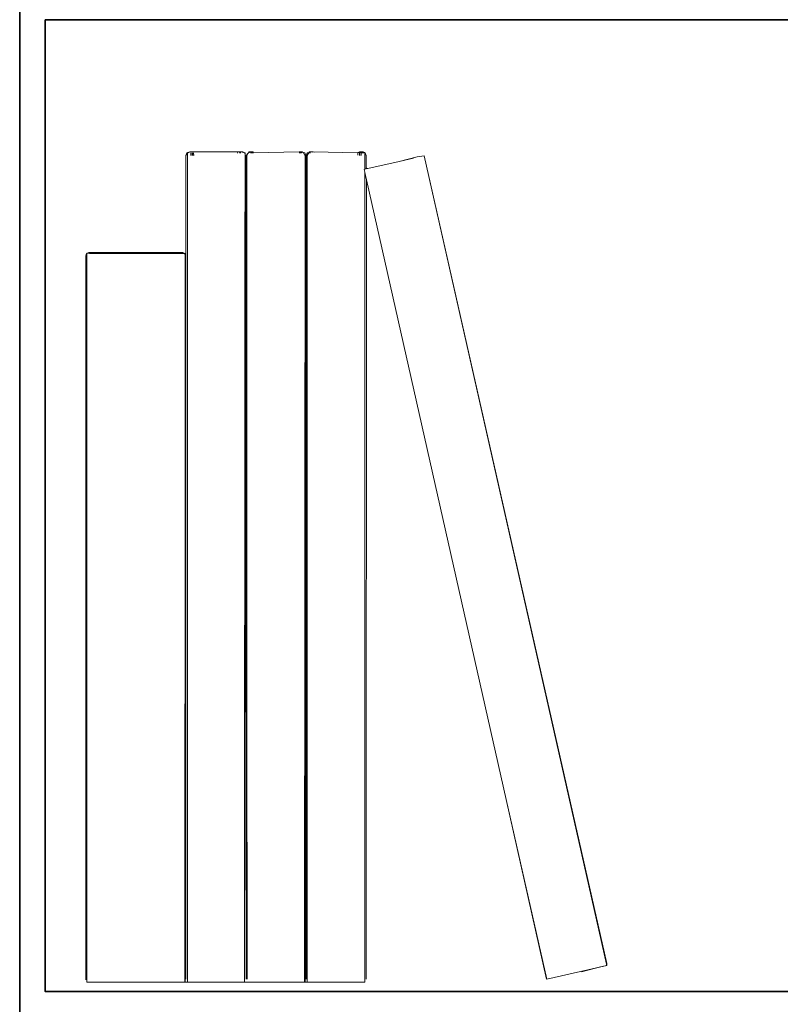
# Model space of a CAD drawing. Units: millimetres. Extents: x 446512 to 447461, y 70395 to 70610.
# Tile 5 of 39: x 446699.43 to 446714.29, y 70453.63 to 70472.88. Entities that reach past the tile are written whole.
import ezdxf

# ---------------------------------------------------------------- set-up
doc = ezdxf.new("R2010")
doc.units = ezdxf.units.MM
doc.layers.add('A-FURN', color=7, linetype='Continuous', lineweight=35)
doc.layers.add('A-FURN-DECO', color=8, linetype='Continuous', lineweight=13)

# ---------------------------------------------------------------- blocks, each defined once
blk = doc.blocks.new('DECO-VASE-C')
for p, q in [((1.958, 16.16), (1.977, 16.215)), ((1.977, 16.202), (1.958, 16.16)), ((1.977, 16.215), (1.982, 16.215)), ((1.977, 16.215), (1.977, 16.202)), ((1.982, 16.215), (1.977, 16.202)), ((1.977, 16.202), (1.977, 16.17)), ((1.982, 16.215), (1.989, 16.215)), ((1.989, 16.215), (1.988, 0)), ((1.989, 16.215), (1.997, 16.218)), ((1.997, 16.218), (2.035, 16.233)), ((2.016, 16.22), (1.997, 16.218)), ((1.997, 16.218), (2.009, 16.215)), ((2.019, 16.221), (2.016, 16.22)), ((3.07, 16.233), (2.035, 16.233)), ((2.054, 16.161), (2.053, 16.215)), ((2.058, 16.161), (2.058, 16.215)), ((2.088, 16.215), (2.094, 16.163)), ((2.088, 16.163), (2.088, 16.215)), ((2.088, 16.215), (2.09, 16.163)), ((2.106, 16.215), (2.11, 16.164)), ((2.969, 16.21), (2.969, 16.215)), ((2.976, 16.215), (2.969, 16.215)), ((2.999, 16.212), (2.999, 16.215)), ((3.004, 16.215), (3.004, 16.212)), ((3.034, 16.215), (3.004, 16.215)), ((3.058, 16.224), (3.11, 16.215)), ((3.07, 16.233), (3.111, 16.215)), ((3.111, 16.215), (3.11, 16.215)), ((3.114, 16.16), (3.111, 16.215)), ((3.115, 16.215), (3.111, 16.215)), ((3.114, 16.16), (3.115, 16.215)), ((3.133, 16.16), (3.177, 16.207)), ((3.152, 16.16), (3.177, 16.207)), ((3.177, 16.207), (3.184, 16.215)), ((3.184, 16.215), (3.19, 16.233)), ((3.184, 16.215), (3.23, 16.225)), ((3.27, 16.233), (3.19, 16.233)), ((3.221, 16.215), (3.263, 16.215)), ((3.263, 16.218), (3.263, 16.215)), ((3.263, 16.215), (3.281, 16.216)), ((3.281, 16.216), (3.27, 16.233)), ((3.281, 16.216), (4.174, 16.232)), ((4.171, 16.215), (4.179, 16.215)), ((4.176, 16.233), (4.174, 16.232)), ((4.178, 16.232), (4.176, 16.233)), ((4.178, 16.232), (4.232, 16.233)), ((4.179, 16.215), (4.179, 16.217)), ((4.209, 16.215), (4.179, 16.215)), ((4.209, 16.215), (4.196, 16.222)), ((4.214, 16.215), (4.209, 16.215)), ((4.212, 16.227), (4.224, 16.225)), ((4.224, 16.225), (4.214, 16.215)), ((4.232, 16.233), (4.224, 16.225)), ((4.224, 16.225), (4.249, 16.221)), ((4.232, 16.233), (4.249, 16.221)), ((4.249, 16.221), (4.258, 16.215)), ((4.249, 16.221), (4.285, 16.215)), ((4.283, 16.171), (4.258, 16.215)), ((4.283, 16.171), (4.285, 16.17)), ((4.29, 16.16), (4.283, 16.171)), ((4.309, 16.16), (4.285, 16.215)), ((4.309, 16.16), (4.327, 16.215)), ((4.332, 16.215), (4.309, 16.16)), ((4.327, 16.215), (4.332, 16.215)), ((4.327, 16.16), (4.36, 16.215)), ((4.332, 16.215), (4.363, 16.22)), ((4.36, 16.215), (4.332, 16.215)), ((4.36, 16.215), (4.363, 16.22)), ((4.396, 16.215), (4.36, 16.215)), ((4.363, 16.22), (4.37, 16.233)), ((4.363, 16.22), (4.384, 16.223)), ((4.439, 16.232), (4.37, 16.233)), ((4.438, 16.212), (4.438, 16.215)), ((4.442, 16.233), (4.439, 16.232)), ((4.439, 16.232), (4.444, 16.232)), ((4.442, 16.233), (4.444, 16.232)), ((4.442, 16.212), (4.442, 16.215)), ((4.444, 16.232), (5.319, 16.215)), ((4.469, 16.211), (4.47, 16.215)), ((5.319, 16.215), (5.317, 16.165)), ((5.319, 16.215), (5.322, 16.217)), ((5.322, 16.217), (5.351, 16.233)), ((5.322, 16.217), (5.35, 16.216)), ((5.35, 16.216), (5.348, 16.163)), ((5.351, 16.233), (5.35, 16.216)), ((5.35, 16.216), (5.354, 16.216)), ((5.351, 16.233), (5.354, 16.216)), ((5.383, 16.215), (5.351, 16.233)), ((5.351, 16.233), (5.422, 16.233)), ((5.351, 16.233), (5.398, 16.222)), ((5.403, 16.224), (5.351, 16.233)), ((5.354, 16.216), (5.352, 16.163)), ((5.354, 16.216), (5.355, 16.163)), ((5.354, 16.216), (5.383, 16.215)), ((5.383, 16.215), (5.386, 16.215)), ((5.383, 16.215), (5.384, 16.215)), ((5.384, 16.161), (5.384, 16.215)), ((5.384, 16.161), (5.386, 16.215)), ((5.384, 16.215), (5.386, 16.215)), ((5.386, 16.215), (5.433, 16.215)), ((5.386, 16.215), (5.388, 16.215)), ((5.388, 16.215), (5.398, 16.222)), ((5.398, 16.222), (5.4, 16.222)), ((5.4, 16.222), (5.403, 16.224)), ((5.4, 16.222), (5.433, 16.215)), ((5.405, 16.224), (5.403, 16.224)), ((5.405, 16.224), (5.422, 16.233)), ((5.449, 16.217), (5.405, 16.224)), ((5.449, 16.217), (5.422, 16.233)), ((5.433, 16.215), (5.449, 16.217)), ((5.453, 16.215), (5.449, 16.217)), ((5.453, 16.215), (5.453, 15.894)), ((5.465, 16.215), (5.453, 16.215)), ((5.465, 16.215), (5.484, 16.16)), ((5.465, 16.17), (5.465, 16.215)), ((1.958, 0.055), (1.958, 16.16)), ((3.114, 16.16), (3.113, 13.969)), ((3.133, 0.055), (3.114, 16.16)), ((3.152, 3.273), (3.133, 16.16)), ((3.133, 16.16), (3.153, 0.055)), ((3.152, 3.273), (3.152, 16.16)), ((4.279, 0), (4.29, 16.16)), ((4.285, 0), (4.309, 16.16)), ((4.29, 0), (4.309, 16.16)), ((4.309, 0.055), (4.309, 16.16)), ((4.309, 16.16), (4.327, 0.012)), ((4.331, 0.004), (4.327, 16.16)), ((5.484, 16.16), (5.484, 15.909)), ((5.516, 15.905), (6.127, 16.043)), ((6.127, 16.043), (6.476, 16.134)), ((6.127, 16.043), (6.409, 16.107)), ((6.614, 16.153), (6.476, 16.134)), ((6.615, 16.153), (6.614, 16.153)), ((6.614, 16.153), (10.177, 0.349)), ((10.188, 0.362), (6.615, 16.153)), ((5.442, 15.889), (5.453, 15.894)), ((5.442, 15.889), (5.454, 15.891)), ((5.453, 15.838), (5.442, 15.889)), ((5.453, 15.894), (5.484, 15.909)), ((5.453, 15.894), (5.454, 15.891)), ((5.453, 15.838), (5.453, 15.829)), ((5.453, 15.829), (5.454, 0)), ((5.485, 15.688), (5.453, 15.829)), ((5.516, 15.905), (5.454, 15.891)), ((5.492, 15.912), (5.484, 15.909)), ((5.484, 15.909), (5.484, 15.903)), ((5.492, 15.912), (5.516, 15.905)), ((5.485, 15.688), (5.484, 0.055)), ((5.485, 15.688), (8.218, 3.572)), ((0, 14.202), (0.014, 14.248)), ((0.014, 14.248), (0.018, 14.248)), ((0.014, 14.248), (0.014, 14.237)), ((0.018, 14.248), (0.014, 14.237)), ((0.018, 14.248), (0.023, 14.248)), ((0.023, 14.248), (0.029, 14.25)), ((0.023, 0), (0.023, 14.248)), ((0.029, 14.25), (0.06, 14.263)), ((0.029, 14.25), (0.066, 14.256)), ((0.074, 14.248), (0.029, 14.25)), ((0.06, 14.263), (0.104, 14.263)), ((0.066, 14.256), (0.06, 14.263)), ((0.066, 14.256), (0.104, 14.263)), ((0.074, 14.248), (0.066, 14.256)), ((0.074, 14.248), (0.094, 14.248)), ((0.094, 14.248), (0.104, 14.26)), ((0.101, 14.248), (0.094, 14.248)), ((0.101, 14.248), (0.104, 14.26)), ((0.101, 14.248), (0.105, 14.248)), ((0.107, 14.263), (0.104, 14.263)), ((0.104, 14.26), (0.104, 14.263)), ((0.105, 14.248), (0.104, 14.26)), ((0.104, 14.26), (0.129, 14.248)), ((0.129, 14.248), (0.105, 14.248)), ((0.129, 14.248), (0.107, 14.263)), ((0.107, 14.263), (1.898, 14.263)), ((1.839, 14.248), (0.129, 14.248)), ((1.842, 14.248), (1.839, 14.248)), ((1.857, 14.248), (1.842, 14.248)), ((1.857, 14.248), (1.898, 14.263)), ((1.857, 14.248), (1.88, 14.248)), ((1.88, 14.248), (1.884, 14.248)), ((1.883, 14.248), (1.88, 14.248)), ((1.884, 14.248), (1.883, 14.248)), ((1.898, 14.263), (1.884, 14.248)), ((1.884, 14.248), (1.89, 14.248)), ((1.89, 14.248), (1.94, 14.248)), ((1.898, 14.263), (1.94, 14.248)), ((1.944, 14.248), (1.94, 14.248)), ((1.943, 14.202), (1.94, 14.248)), ((1.943, 14.202), (1.944, 14.248)), ((0.014, 14.237), (0, 14.202)), ((0, 0.043), (0, 14.202)), ((0.014, 14.237), (0.014, 14.21)), ((1.943, 14.202), (1.941, 13.498)), ((1.958, 0.055), (1.943, 14.202)), ((3.113, 13.969), (3.104, 0)), ((3.113, 13.969), (3.133, 0.055)), ((1.941, 13.498), (1.944, 10.898)), ((1.944, 10.898), (1.935, 0)), ((1.944, 10.898), (1.958, 0.055)), ((1.945, 0.01), (1.944, 10.898)), ((8.218, 3.572), (9.007, 0.059)), ((9.01, 0.059), (8.218, 3.572)), ((10.183, 0.324), (9.01, 0.058)), ((10.06, 0.296), (9.693, 0.201)), ((10.06, 0.296), (10.181, 0.323)), ((10.183, 0.324), (10.177, 0.349)), ((10.177, 0.349), (10.181, 0.323)), ((10.183, 0.324), (10.181, 0.323)), ((10.188, 0.362), (10.183, 0.324)), ((0.023, 0), (5.454, 0))]:
    blk.add_line(p, q)

msp = doc.modelspace()

# ---------------------------------------------------------------- linework, layer by layer
at = {"layer": 'A-FURN'}
msp.add_line((446699.4288, 70473.3815), (446699.4288, 70453.3815), dxfattribs=at)
for points in [[(446699.4288, 70473.3815), (446746.5728, 70473.3815), (446746.5728, 70453.3815), (446699.4288, 70453.3815)], [(446699.9288, 70472.8815), (446746.0728, 70472.8815), (446746.0728, 70453.8815), (446699.9288, 70453.8815)]]:
    msp.add_lwpolyline(points, close=True, dxfattribs=at)

# ---------------------------------------------------------------- block references
at = {"layer": 'A-FURN-DECO'}
msp.add_blockref('DECO-VASE-C', (446700.719, 70454.065), dxfattribs=at)

doc.saveas('drawing.dxf')
